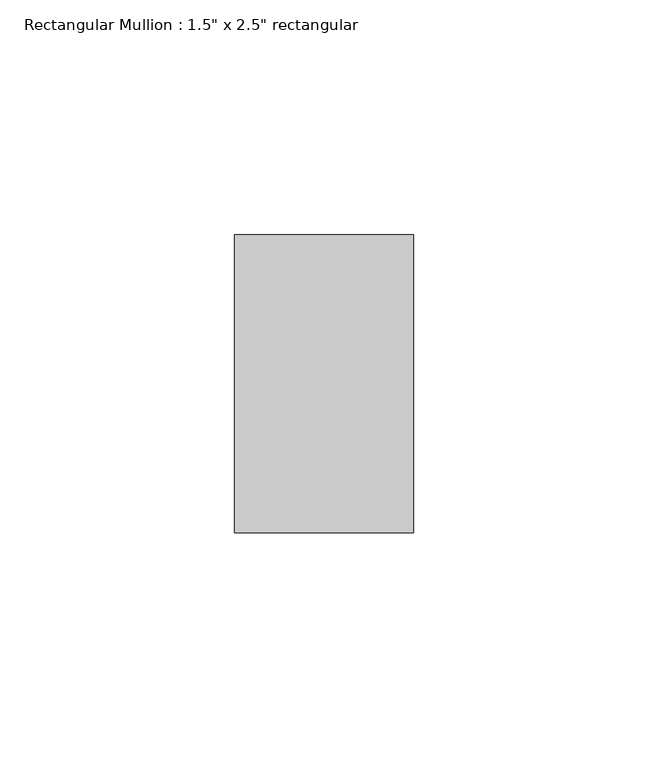
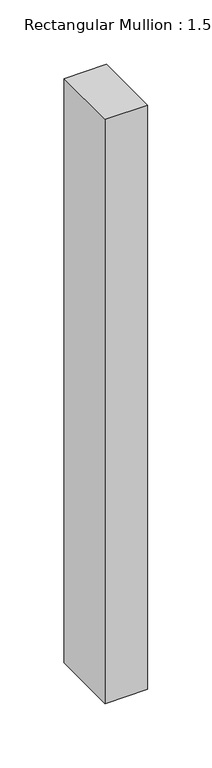
"""IFC4 building model written with IfcOpenShell, lengths in millimetres: member geometry."""

from ifc_helpers import new_model, si_unit, frame, origin, place, context, project, spatial, polyline, outline, extrude, source, transform, mapped, element, save


def member_c8158400(model_context):
    return source(origin(), model_context, "Body", "SweptSolid", [
        extrude(outline(polyline([(0.0, 31.75), (0.0, -31.75), (-38.1, -31.75), (-38.1, 31.75), (0.0, 31.75)])), frame((0.0, 0.0, -553.3665215), z_axis=(0.0, 0.0, 1.0), x_axis=(1.0, 0.0, 0.0)), (0.0, 0.0, 1.0), 553.3665215),
    ])


if __name__ == "__main__":
    model = new_model("IFC4")
    model_context = context("Model", 3, world=origin())
    ifc_project = project(units=[si_unit("LENGTHUNIT", "METRE", prefix="MILLI")], contexts=[model_context])
    site = spatial("IfcSite", under=ifc_project)
    building = spatial("IfcBuilding", under=site)
    placement = place(None, origin())
    member_shape = member_c8158400(model_context)
    element("IfcMember", 1, ObjectType="Rectangular Mullion : 1.5\" x 2.5\" rectangular", at=placement, inside=building, context=model_context, shape_type="MappedRepresentation", body=[
        mapped(member_shape, transform((0.0, 0.0, 0.0), x_axis=(1.0, 0.0, 0.0), y_axis=(0.0, 1.0, 0.0), z_axis=(0.0, 0.0, 1.0))),
    ])
    save(model, "model.ifc")

# Revit data of these elements
# Type "Rectangular Mullion : 1.5\" x 2.5\" rectangular"
#   built-in parameter 1007304 = 0.208333 (stored number, unit not read)
#   built-in parameter 1007301 = 0.0625 (stored number, unit not read)
#   built-in parameter 1007300 = 0.0625 (stored number, unit not read)
